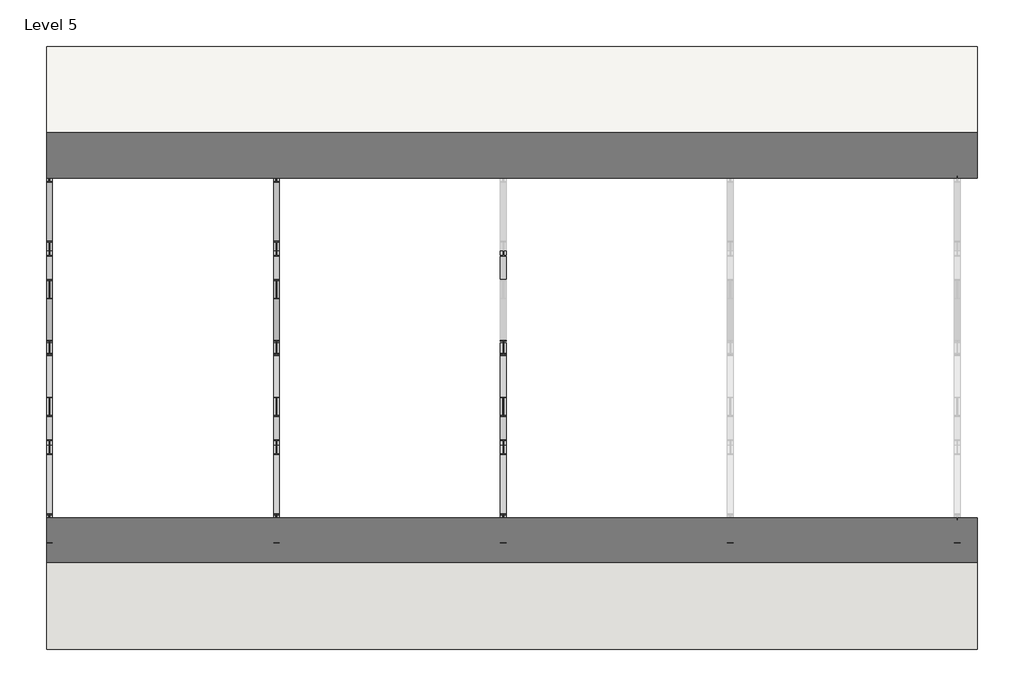
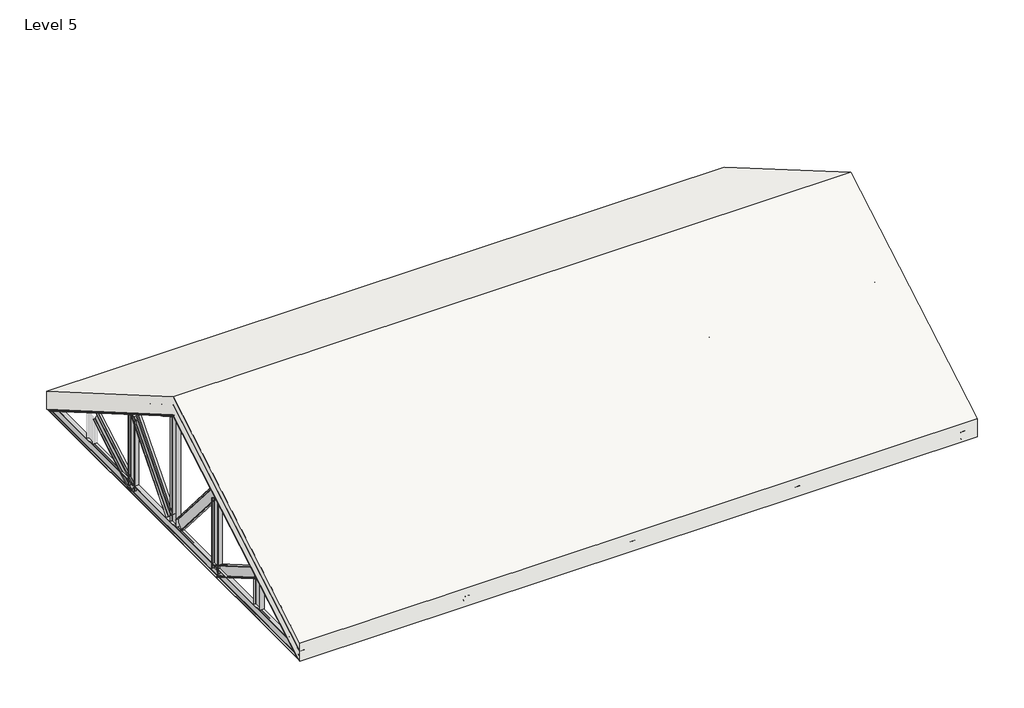
# One storey, part 1 of 2: 29 beams, 1 roof.
"""IFC4 building model written with IfcOpenShell, lengths in millimetres."""

from ifc_helpers import new_model, si_unit, frame, origin, place, context, project, spatial, polyline, circle_curve, ellipse_curve, outline, extrude, transform, mapped, element, save
from ifc_brep_helpers import plane_surface, revolved_surface, advanced_brep
from components import ub_universal_beams_ub254x102x28_e74905dc, ub_universal_beams_ub254x102x28_1dca85a9, ub_universal_beams_ub254x102x28_3582687b, ub_universal_beams_ub254x102x28_9eef3cd1, ub_universal_beams_ub254x102x28_f7ef6108, ub_universal_beams_ub254x102x28_93a23aa5, ub_universal_beams_ub254x102x28_1ec9d6d8, ub_universal_beams_ub254x102x28_a06fb1b7

model = new_model("IFC4")

# Units and contexts
model_context = context("Model", 3, world=origin())
ifc_project = project(units=[si_unit("LENGTHUNIT", "METRE", prefix="MILLI")], contexts=[model_context])

# Site, building, storey
site = spatial("IfcSite", under=ifc_project)
building = spatial("IfcBuilding", under=site)
storey = spatial("IfcBuildingStorey", under=building, Name="Level 5", Elevation=9144.0)

# Beams
placement = place(None, origin())
element("IfcBeam", 1, ObjectType="UB-Universal Beams : UB254x102x28", at=placement, inside=storey, context=model_context, shape_type="AdvancedBrep", body=[
    advanced_brep(
    [(-8879.5620752, 9795.4298445, 9040.0618528), (-8879.5620752, 9790.4089662, 9031.4136864), (-8981.7620752, 9790.4089662, 9031.4136864), (-8981.7620752, 9795.4298445, 9040.0618528), (-8941.4120752, 9795.4298445, 9040.0618528), (-8933.8120752, 9799.245712, 9046.6344592), (-8933.8120752, 9912.3158911, 9241.3911653), (-8941.4120752, 9916.1317586, 9247.9637718), (-8981.7620752, 9916.1317586, 9247.9637718), (-8981.7620752, 9921.1526369, 9256.6119381), (-8879.5620752, 9921.1526369, 9256.6119381), (-8879.5620752, 9916.1317586, 9247.9637718), (-8919.9120752, 9916.1317586, 9247.9637718), (-8927.5120752, 9912.3158911, 9241.3911653), (-8927.5120752, 9799.245712, 9046.6344592), (-8919.9120752, 9795.4298445, 9040.0618528), (-8919.9120752, 4605.8028699, 12053.0109991), (-8879.5620752, 4605.8028699, 12053.0109991), (-8927.5120752, 4605.8028699, 12061.7989892), (-8927.5120752, 4605.8028699, 12322.2010108), (-8919.9120752, 4605.8028699, 12330.9890009), (-8879.5620752, 4605.8028699, 12330.9890009), (-8879.5620752, 4605.8028699, 12342.5521457), (-8981.7620752, 4605.8028699, 12342.5521457), (-8981.7620752, 4605.8028699, 12330.9890009), (-8941.4120752, 4605.8028699, 12330.9890009), (-8933.8120752, 4605.8028699, 12322.2010108), (-8933.8120752, 4605.8028699, 12061.7989892), (-8941.4120752, 4605.8028699, 12053.0109991), (-8981.7620752, 4605.8028699, 12053.0109991), (-8981.7620752, 4605.8028699, 12041.4478543), (-8879.5620752, 4605.8028699, 12041.4478543)],
    [
        (0, 1),
        (1, 2),
        (2, 3),
        (3, 4),
        (4, 5, circle_curve(frame((-8941.4120752, 9799.245712, 9046.6344592), z_axis=(0.0, -0.8648166348106393, 0.5020878291243489), x_axis=(-1.0, 0.0, 0.0)), 7.6)),
        (5, 6),
        (6, 7, circle_curve(frame((-8941.4120752, 9912.3158911, 9241.3911653), z_axis=(0.0, -0.8648166348106393, 0.5020878291243489), x_axis=(-1.0, 0.0, 0.0)), 7.6)),
        (7, 8),
        (8, 9),
        (9, 10),
        (10, 11),
        (11, 12),
        (12, 13, circle_curve(frame((-8919.9120752, 9912.3158911, 9241.3911653), z_axis=(0.0, -0.8648166348106393, 0.5020878291243489), x_axis=(-1.0, 0.0, 0.0)), 7.6)),
        (13, 14),
        (14, 15, circle_curve(frame((-8919.9120752, 9799.245712, 9046.6344592), z_axis=(0.0, -0.8648166348106393, 0.5020878291243489), x_axis=(-1.0, 0.0, 0.0)), 7.6)),
        (15, 0),
        (16, 17),
        (17, 0),
        (15, 16),
        (18, 16, ellipse_curve(frame((-8919.9120752, 4605.8028699, 12061.7989892), z_axis=(0.0, -1.0, 0.0), x_axis=(0.0, 0.0, -1.0)), 8.7879901, 7.6)),
        (14, 18),
        (19, 18),
        (13, 19),
        (20, 19, ellipse_curve(frame((-8919.9120752, 4605.8028699, 12322.2010108), z_axis=(0.0, -1.0, 0.0), x_axis=(0.0, 0.0, -1.0)), 8.7879901, 7.6)),
        (12, 20),
        (21, 20),
        (11, 21),
        (22, 21),
        (10, 22),
        (23, 22),
        (9, 23),
        (24, 23),
        (8, 24),
        (25, 24),
        (7, 25),
        (26, 25, ellipse_curve(frame((-8941.4120752, 4605.8028699, 12322.2010108), z_axis=(0.0, -1.0, 0.0), x_axis=(0.0, 0.0, -1.0)), 8.7879901, 7.6)),
        (6, 26),
        (27, 26),
        (5, 27),
        (28, 27, ellipse_curve(frame((-8941.4120752, 4605.8028699, 12061.7989892), z_axis=(0.0, -1.0, 0.0), x_axis=(0.0, 0.0, -1.0)), 8.7879901, 7.6)),
        (4, 28),
        (29, 28),
        (3, 29),
        (30, 29),
        (2, 30),
        (31, 30),
        (1, 31),
        (17, 31),
    ],
    [
        plane_surface(frame((-8930.6620752, 9855.7808016, 9144.0128123), z_axis=(0.0, 0.8648166348106393, -0.5020878291243489), x_axis=(0.0, 0.5020878291243489, 0.8648166348106393))),
        plane_surface(frame((-8879.5620752, 4545.4739812, 12088.0362282), z_axis=(0.0, 0.5020878291243489, 0.8648166348106393), x_axis=(0.0, 0.8648166348106393, -0.5020878291243489))),
        revolved_surface(polyline([(-8927.5120752, 9799.245712003027, 9046.634459205212), (-8927.5120752, 4601.987002407376, 12064.01437289046)]), (-8919.9120752, 4549.2898487, 12094.6088347), (0.0, 0.8648166348106393, -0.5020878291243489)),
        plane_surface(frame((-8927.5120752, 4549.2898487, 12094.6088347), z_axis=(1.0, 0.0, 0.0), x_axis=(0.0, 0.8648166348106393, -0.5020878291243489))),
        revolved_surface(polyline([(-8927.5120752, 9912.315891103026, 9241.391165305211), (-8927.5120752, 4601.987002367825, 12324.416394422336)]), (-8919.9120752, 4662.3600278, 12289.3655408), (0.0, 0.8648166348106393, -0.5020878291243489)),
        plane_surface(frame((-8919.9120752, 4666.1758953, 12295.9381472), z_axis=(0.0, -0.5020878291243489, -0.8648166348106393), x_axis=(0.0, 0.8648166348106393, -0.5020878291243489))),
        plane_surface(frame((-8879.5620752, 4666.1758953, 12295.9381472), z_axis=(1.0, 0.0, 0.0), x_axis=(0.0, 0.8648166348106393, -0.5020878291243489))),
        plane_surface(frame((-8879.5620752, 4671.1967736, 12304.5863136), z_axis=(0.0, 0.5020878291243489, 0.8648166348106393), x_axis=(0.0, 0.8648166348106393, -0.5020878291243489))),
        plane_surface(frame((-8981.7620752, 4671.1967736, 12304.5863136), z_axis=(-1.0, 0.0, 0.0), x_axis=(0.0, 0.8648166348106393, -0.5020878291243489))),
        plane_surface(frame((-8981.7620752, 4666.1758953, 12295.9381472), z_axis=(0.0, -0.5020878291243489, -0.8648166348106393), x_axis=(0.0, 0.8648166348106393, -0.5020878291243489))),
        revolved_surface(polyline([(-8949.0120752, 9912.315891103026, 9241.391165305211), (-8949.0120752, 4601.987002367825, 12324.416394422336)]), (-8941.4120752, 4662.3600278, 12289.3655408), (0.0, 0.8648166348106393, -0.5020878291243489)),
        plane_surface(frame((-8933.8120752, 4662.3600278, 12289.3655408), z_axis=(-1.0, 0.0, 0.0), x_axis=(0.0, 0.8648166348106393, -0.5020878291243489))),
        revolved_surface(polyline([(-8949.0120752, 9799.245712003027, 9046.634459205212), (-8949.0120752, 4601.987002407376, 12064.01437289046)]), (-8941.4120752, 4549.2898487, 12094.6088347), (0.0, 0.8648166348106393, -0.5020878291243489)),
        plane_surface(frame((-8941.4120752, 4545.4739812, 12088.0362282), z_axis=(0.0, 0.5020878291243489, 0.8648166348106393), x_axis=(0.0, 0.8648166348106393, -0.5020878291243489))),
        plane_surface(frame((-8981.7620752, 4545.4739812, 12088.0362282), z_axis=(-1.0, 0.0, 0.0), x_axis=(0.0, 0.8648166348106393, -0.5020878291243489))),
        plane_surface(frame((-8981.7620752, 4540.4531029, 12079.3880619), z_axis=(0.0, -0.5020878291243489, -0.8648166348106393), x_axis=(0.0, 0.8648166348106393, -0.5020878291243489))),
        plane_surface(frame((-8879.5620752, 4540.4531029, 12079.3880619), z_axis=(1.0, 0.0, 0.0), x_axis=(0.0, 0.8648166348106393, -0.5020878291243489))),
        plane_surface(frame((-8930.6620752, 4605.8028699, 12342.5521457), z_axis=(0.0, -1.0, 0.0), x_axis=(0.0, 0.0, 1.0))),
    ],
    [
        (0, [[1, 2, 3, 4, 5, 6, 7, 8, 9, 10, 11, 12, 13, 14, 15, 16]]),
        (1, [[17, 18, -16, 19]]),
        (2, [[20, -19, -15, 21]]),
        (3, [[22, -21, -14, 23]]),
        (4, [[24, -23, -13, 25]]),
        (5, [[26, -25, -12, 27]]),
        (6, [[28, -27, -11, 29]]),
        (7, [[30, -29, -10, 31]]),
        (8, [[32, -31, -9, 33]]),
        (9, [[34, -33, -8, 35]]),
        (10, [[36, -35, -7, 37]]),
        (11, [[38, -37, -6, 39]]),
        (12, [[40, -39, -5, 41]]),
        (13, [[42, -41, -4, 43]]),
        (14, [[44, -43, -3, 45]]),
        (15, [[46, -45, -2, 47]]),
        (16, [[48, -47, -1, -18]]),
        (17, [[-17, -20, -22, -24, -26, -28, -30, -32, -34, -36, -38, -40, -42, -44, -46, -48]]),
    ],
),
])
element("IfcBeam", 2, ObjectType="UB-Universal Beams : UB254x102x28", at=placement, inside=storey, context=model_context, shape_type="AdvancedBrep", body=[
    advanced_brep(
    [(-8879.5620752, -583.8241047, 9040.0618528), (-8919.9120752, -583.8241047, 9040.0618528), (-8927.5120752, -587.6399722, 9046.6344592), (-8927.5120752, -700.7101513, 9241.3911653), (-8919.9120752, -704.5260188, 9247.9637718), (-8879.5620752, -704.5260188, 9247.9637718), (-8879.5620752, -709.5468971, 9256.6119381), (-8981.7620752, -709.5468971, 9256.6119381), (-8981.7620752, -704.5260188, 9247.9637718), (-8941.4120752, -704.5260188, 9247.9637718), (-8933.8120752, -700.7101513, 9241.3911653), (-8933.8120752, -587.6399722, 9046.6344592), (-8941.4120752, -583.8241047, 9040.0618528), (-8981.7620752, -583.8241047, 9040.0618528), (-8981.7620752, -578.8032264, 9031.4136864), (-8879.5620752, -578.8032264, 9031.4136864), (-8879.5620752, 4605.8028699, 12053.0109991), (-8919.9120752, 4605.8028699, 12053.0109991), (-8927.5120752, 4605.8028699, 12061.7989892), (-8927.5120752, 4605.8028699, 12322.2010108), (-8919.9120752, 4605.8028699, 12330.9890009), (-8879.5620752, 4605.8028699, 12330.9890009), (-8879.5620752, 4605.8028699, 12342.5521457), (-8981.7620752, 4605.8028699, 12342.5521457), (-8981.7620752, 4605.8028699, 12330.9890009), (-8941.4120752, 4605.8028699, 12330.9890009), (-8933.8120752, 4605.8028699, 12322.2010108), (-8933.8120752, 4605.8028699, 12061.7989892), (-8941.4120752, 4605.8028699, 12053.0109991), (-8981.7620752, 4605.8028699, 12053.0109991), (-8981.7620752, 4605.8028699, 12041.4478543), (-8879.5620752, 4605.8028699, 12041.4478543)],
    [
        (0, 1),
        (1, 2, circle_curve(frame((-8919.9120752, -587.6399722, 9046.6344592), z_axis=(0.0, 0.8648166348106395, 0.5020878291243485), x_axis=(-1.0, 0.0, 0.0)), 7.6)),
        (2, 3),
        (3, 4, circle_curve(frame((-8919.9120752, -700.7101513, 9241.3911653), z_axis=(0.0, 0.8648166348106395, 0.5020878291243485), x_axis=(-1.0, 0.0, 0.0)), 7.6)),
        (4, 5),
        (5, 6),
        (6, 7),
        (7, 8),
        (8, 9),
        (9, 10, circle_curve(frame((-8941.4120752, -700.7101513, 9241.3911653), z_axis=(0.0, 0.8648166348106395, 0.5020878291243485), x_axis=(-1.0, 0.0, 0.0)), 7.6)),
        (10, 11),
        (11, 12, circle_curve(frame((-8941.4120752, -587.6399722, 9046.6344592), z_axis=(0.0, 0.8648166348106395, 0.5020878291243485), x_axis=(-1.0, 0.0, 0.0)), 7.6)),
        (12, 13),
        (13, 14),
        (14, 15),
        (15, 0),
        (0, 16),
        (16, 17),
        (17, 1),
        (17, 18, ellipse_curve(frame((-8919.9120752, 4605.8028699, 12061.7989892), z_axis=(0.0, 1.0, 0.0), x_axis=(0.0, 0.0, 1.0)), 8.7879901, 7.6)),
        (18, 2),
        (18, 19),
        (19, 3),
        (19, 20, ellipse_curve(frame((-8919.9120752, 4605.8028699, 12322.2010108), z_axis=(0.0, 1.0, 0.0), x_axis=(0.0, 0.0, 1.0)), 8.7879901, 7.6)),
        (20, 4),
        (20, 21),
        (21, 5),
        (21, 22),
        (22, 6),
        (22, 23),
        (23, 7),
        (23, 24),
        (24, 8),
        (24, 25),
        (25, 9),
        (25, 26, ellipse_curve(frame((-8941.4120752, 4605.8028699, 12322.2010108), z_axis=(0.0, 1.0, 0.0), x_axis=(0.0, 0.0, 1.0)), 8.7879901, 7.6)),
        (26, 10),
        (26, 27),
        (27, 11),
        (27, 28, ellipse_curve(frame((-8941.4120752, 4605.8028699, 12061.7989892), z_axis=(0.0, 1.0, 0.0), x_axis=(0.0, 0.0, 1.0)), 8.7879901, 7.6)),
        (28, 12),
        (28, 29),
        (29, 13),
        (29, 30),
        (30, 14),
        (30, 31),
        (31, 15),
        (31, 16),
    ],
    [
        plane_surface(frame((-8930.6620752, -644.1750617, 9144.0128123), z_axis=(0.0, -0.8648166348106395, -0.5020878291243485), x_axis=(0.0, -0.5020878291243485, 0.8648166348106395))),
        plane_surface(frame((-8879.5620752, -583.8241047, 9040.0618528), z_axis=(0.0, -0.5020878291243485, 0.8648166348106395), x_axis=(0.0, 0.8648166348106395, 0.5020878291243485))),
        revolved_surface(polyline([(-8927.5120752, 4609.618737395652, 12064.014372885247), (-8927.5120752, -587.6399722, 9046.6344592)]), (-8919.9120752, -587.6399722, 9046.6344592), (0.0, 0.8648166348106395, 0.5020878291243485)),
        plane_surface(frame((-8927.5120752, -587.6399722, 9046.6344592), z_axis=(1.0, 0.0, 0.0), x_axis=(0.0, 0.8648166348106395, 0.5020878291243485))),
        revolved_surface(polyline([(-8927.5120752, 4609.618737435201, 12324.416394417123), (-8927.5120752, -700.7101513, 9241.3911653)]), (-8919.9120752, -700.7101513, 9241.3911653), (0.0, 0.8648166348106395, 0.5020878291243485)),
        plane_surface(frame((-8919.9120752, -704.5260188, 9247.9637718), z_axis=(0.0, 0.5020878291243485, -0.8648166348106395), x_axis=(0.0, 0.8648166348106395, 0.5020878291243485))),
        plane_surface(frame((-8879.5620752, -704.5260188, 9247.9637718), z_axis=(1.0, 0.0, 0.0), x_axis=(0.0, 0.8648166348106395, 0.5020878291243485))),
        plane_surface(frame((-8879.5620752, -709.5468971, 9256.6119381), z_axis=(0.0, -0.5020878291243485, 0.8648166348106395), x_axis=(0.0, 0.8648166348106395, 0.5020878291243485))),
        plane_surface(frame((-8981.7620752, -709.5468971, 9256.6119381), z_axis=(-1.0, 0.0, 0.0), x_axis=(0.0, 0.8648166348106395, 0.5020878291243485))),
        plane_surface(frame((-8981.7620752, -704.5260188, 9247.9637718), z_axis=(0.0, 0.5020878291243485, -0.8648166348106395), x_axis=(0.0, 0.8648166348106395, 0.5020878291243485))),
        revolved_surface(polyline([(-8949.0120752, 4609.618737435201, 12324.416394417123), (-8949.0120752, -700.7101513, 9241.3911653)]), (-8941.4120752, -700.7101513, 9241.3911653), (0.0, 0.8648166348106395, 0.5020878291243485)),
        plane_surface(frame((-8933.8120752, -700.7101513, 9241.3911653), z_axis=(-1.0, 0.0, 0.0), x_axis=(0.0, 0.8648166348106395, 0.5020878291243485))),
        revolved_surface(polyline([(-8949.0120752, 4609.618737395652, 12064.014372885247), (-8949.0120752, -587.6399722, 9046.6344592)]), (-8941.4120752, -587.6399722, 9046.6344592), (0.0, 0.8648166348106395, 0.5020878291243485)),
        plane_surface(frame((-8941.4120752, -583.8241047, 9040.0618528), z_axis=(0.0, -0.5020878291243485, 0.8648166348106395), x_axis=(0.0, 0.8648166348106395, 0.5020878291243485))),
        plane_surface(frame((-8981.7620752, -583.8241047, 9040.0618528), z_axis=(-1.0, 0.0, 0.0), x_axis=(0.0, 0.8648166348106395, 0.5020878291243485))),
        plane_surface(frame((-8981.7620752, -578.8032264, 9031.4136864), z_axis=(0.0, 0.5020878291243485, -0.8648166348106395), x_axis=(0.0, 0.8648166348106395, 0.5020878291243485))),
        plane_surface(frame((-8879.5620752, -578.8032264, 9031.4136864), z_axis=(1.0, 0.0, 0.0), x_axis=(0.0, 0.8648166348106395, 0.5020878291243485))),
        plane_surface(frame((-8930.6620752, 4605.8028699, 12342.5521457), z_axis=(0.0, 1.0, 0.0), x_axis=(0.0, 0.0, -1.0))),
    ],
    [
        (0, [[1, 2, 3, 4, 5, 6, 7, 8, 9, 10, 11, 12, 13, 14, 15, 16]]),
        (1, [[-1, 17, 18, 19]]),
        (2, [[-2, -19, 20, 21]]),
        (3, [[-3, -21, 22, 23]]),
        (4, [[-4, -23, 24, 25]]),
        (5, [[-5, -25, 26, 27]]),
        (6, [[-6, -27, 28, 29]]),
        (7, [[-7, -29, 30, 31]]),
        (8, [[-8, -31, 32, 33]]),
        (9, [[-9, -33, 34, 35]]),
        (10, [[-10, -35, 36, 37]]),
        (11, [[-11, -37, 38, 39]]),
        (12, [[-12, -39, 40, 41]]),
        (13, [[-13, -41, 42, 43]]),
        (14, [[-14, -43, 44, 45]]),
        (15, [[-15, -45, 46, 47]]),
        (16, [[-16, -47, 48, -17]]),
        (17, [[-48, -46, -44, -42, -40, -38, -36, -34, -32, -30, -28, -26, -24, -22, -20, -18]]),
    ],
),
])
element("IfcBeam", 3, ObjectType="UB-Universal Beams : UB254x102x28", at=placement, inside=storey, context=model_context, shape_type="AdvancedBrep", body=[
    advanced_brep(
    [(-4879.5620752, 9795.4298445, 9040.0618528), (-4879.5620752, 9790.4089662, 9031.4136864), (-4981.7620752, 9790.4089662, 9031.4136864), (-4981.7620752, 9795.4298445, 9040.0618528), (-4941.4120752, 9795.4298445, 9040.0618528), (-4933.8120752, 9799.245712, 9046.6344592), (-4933.8120752, 9912.3158911, 9241.3911653), (-4941.4120752, 9916.1317586, 9247.9637718), (-4981.7620752, 9916.1317586, 9247.9637718), (-4981.7620752, 9921.1526369, 9256.6119381), (-4879.5620752, 9921.1526369, 9256.6119381), (-4879.5620752, 9916.1317586, 9247.9637718), (-4919.9120752, 9916.1317586, 9247.9637718), (-4927.5120752, 9912.3158911, 9241.3911653), (-4927.5120752, 9799.245712, 9046.6344592), (-4919.9120752, 9795.4298445, 9040.0618528), (-4919.9120752, 4605.8028699, 12053.0109991), (-4879.5620752, 4605.8028699, 12053.0109991), (-4927.5120752, 4605.8028699, 12061.7989892), (-4927.5120752, 4605.8028699, 12322.2010108), (-4919.9120752, 4605.8028699, 12330.9890009), (-4879.5620752, 4605.8028699, 12330.9890009), (-4879.5620752, 4605.8028699, 12342.5521457), (-4981.7620752, 4605.8028699, 12342.5521457), (-4981.7620752, 4605.8028699, 12330.9890009), (-4941.4120752, 4605.8028699, 12330.9890009), (-4933.8120752, 4605.8028699, 12322.2010108), (-4933.8120752, 4605.8028699, 12061.7989892), (-4941.4120752, 4605.8028699, 12053.0109991), (-4981.7620752, 4605.8028699, 12053.0109991), (-4981.7620752, 4605.8028699, 12041.4478543), (-4879.5620752, 4605.8028699, 12041.4478543)],
    [
        (0, 1),
        (1, 2),
        (2, 3),
        (3, 4),
        (4, 5, circle_curve(frame((-4941.4120752, 9799.245712, 9046.6344592), z_axis=(0.0, -0.8648166348106393, 0.5020878291243489), x_axis=(-1.0, 0.0, 0.0)), 7.6)),
        (5, 6),
        (6, 7, circle_curve(frame((-4941.4120752, 9912.3158911, 9241.3911653), z_axis=(0.0, -0.8648166348106393, 0.5020878291243489), x_axis=(-1.0, 0.0, 0.0)), 7.6)),
        (7, 8),
        (8, 9),
        (9, 10),
        (10, 11),
        (11, 12),
        (12, 13, circle_curve(frame((-4919.9120752, 9912.3158911, 9241.3911653), z_axis=(0.0, -0.8648166348106393, 0.5020878291243489), x_axis=(-1.0, 0.0, 0.0)), 7.6)),
        (13, 14),
        (14, 15, circle_curve(frame((-4919.9120752, 9799.245712, 9046.6344592), z_axis=(0.0, -0.8648166348106393, 0.5020878291243489), x_axis=(-1.0, 0.0, 0.0)), 7.6)),
        (15, 0),
        (16, 17),
        (17, 0),
        (15, 16),
        (18, 16, ellipse_curve(frame((-4919.9120752, 4605.8028699, 12061.7989892), z_axis=(0.0, -1.0, 0.0), x_axis=(0.0, 0.0, -1.0)), 8.7879901, 7.6)),
        (14, 18),
        (19, 18),
        (13, 19),
        (20, 19, ellipse_curve(frame((-4919.9120752, 4605.8028699, 12322.2010108), z_axis=(0.0, -1.0, 0.0), x_axis=(0.0, 0.0, -1.0)), 8.7879901, 7.6)),
        (12, 20),
        (21, 20),
        (11, 21),
        (22, 21),
        (10, 22),
        (23, 22),
        (9, 23),
        (24, 23),
        (8, 24),
        (25, 24),
        (7, 25),
        (26, 25, ellipse_curve(frame((-4941.4120752, 4605.8028699, 12322.2010108), z_axis=(0.0, -1.0, 0.0), x_axis=(0.0, 0.0, -1.0)), 8.7879901, 7.6)),
        (6, 26),
        (27, 26),
        (5, 27),
        (28, 27, ellipse_curve(frame((-4941.4120752, 4605.8028699, 12061.7989892), z_axis=(0.0, -1.0, 0.0), x_axis=(0.0, 0.0, -1.0)), 8.7879901, 7.6)),
        (4, 28),
        (29, 28),
        (3, 29),
        (30, 29),
        (2, 30),
        (31, 30),
        (1, 31),
        (17, 31),
    ],
    [
        plane_surface(frame((-4930.6620752, 9855.7808016, 9144.0128123), z_axis=(0.0, 0.8648166348106393, -0.5020878291243489), x_axis=(0.0, 0.5020878291243489, 0.8648166348106393))),
        plane_surface(frame((-4879.5620752, 4545.4739812, 12088.0362282), z_axis=(0.0, 0.5020878291243489, 0.8648166348106393), x_axis=(0.0, 0.8648166348106393, -0.5020878291243489))),
        revolved_surface(polyline([(-4927.5120752, 9799.245712003027, 9046.634459205212), (-4927.5120752, 4601.987002407376, 12064.01437289046)]), (-4919.9120752, 4549.2898487, 12094.6088347), (0.0, 0.8648166348106393, -0.5020878291243489)),
        plane_surface(frame((-4927.5120752, 4549.2898487, 12094.6088347), z_axis=(1.0, 0.0, 0.0), x_axis=(0.0, 0.8648166348106393, -0.5020878291243489))),
        revolved_surface(polyline([(-4927.5120752, 9912.315891103026, 9241.391165305211), (-4927.5120752, 4601.987002367825, 12324.416394422336)]), (-4919.9120752, 4662.3600278, 12289.3655408), (0.0, 0.8648166348106393, -0.5020878291243489)),
        plane_surface(frame((-4919.9120752, 4666.1758953, 12295.9381472), z_axis=(0.0, -0.5020878291243489, -0.8648166348106393), x_axis=(0.0, 0.8648166348106393, -0.5020878291243489))),
        plane_surface(frame((-4879.5620752, 4666.1758953, 12295.9381472), z_axis=(1.0, 0.0, 0.0), x_axis=(0.0, 0.8648166348106393, -0.5020878291243489))),
        plane_surface(frame((-4879.5620752, 4671.1967736, 12304.5863136), z_axis=(0.0, 0.5020878291243489, 0.8648166348106393), x_axis=(0.0, 0.8648166348106393, -0.5020878291243489))),
        plane_surface(frame((-4981.7620752, 4671.1967736, 12304.5863136), z_axis=(-1.0, 0.0, 0.0), x_axis=(0.0, 0.8648166348106393, -0.5020878291243489))),
        plane_surface(frame((-4981.7620752, 4666.1758953, 12295.9381472), z_axis=(0.0, -0.5020878291243489, -0.8648166348106393), x_axis=(0.0, 0.8648166348106393, -0.5020878291243489))),
        revolved_surface(polyline([(-4949.0120752, 9912.315891103026, 9241.391165305211), (-4949.0120752, 4601.987002367825, 12324.416394422336)]), (-4941.4120752, 4662.3600278, 12289.3655408), (0.0, 0.8648166348106393, -0.5020878291243489)),
        plane_surface(frame((-4933.8120752, 4662.3600278, 12289.3655408), z_axis=(-1.0, 0.0, 0.0), x_axis=(0.0, 0.8648166348106393, -0.5020878291243489))),
        revolved_surface(polyline([(-4949.0120752, 9799.245712003027, 9046.634459205212), (-4949.0120752, 4601.987002407376, 12064.01437289046)]), (-4941.4120752, 4549.2898487, 12094.6088347), (0.0, 0.8648166348106393, -0.5020878291243489)),
        plane_surface(frame((-4941.4120752, 4545.4739812, 12088.0362282), z_axis=(0.0, 0.5020878291243489, 0.8648166348106393), x_axis=(0.0, 0.8648166348106393, -0.5020878291243489))),
        plane_surface(frame((-4981.7620752, 4545.4739812, 12088.0362282), z_axis=(-1.0, 0.0, 0.0), x_axis=(0.0, 0.8648166348106393, -0.5020878291243489))),
        plane_surface(frame((-4981.7620752, 4540.4531029, 12079.3880619), z_axis=(0.0, -0.5020878291243489, -0.8648166348106393), x_axis=(0.0, 0.8648166348106393, -0.5020878291243489))),
        plane_surface(frame((-4879.5620752, 4540.4531029, 12079.3880619), z_axis=(1.0, 0.0, 0.0), x_axis=(0.0, 0.8648166348106393, -0.5020878291243489))),
        plane_surface(frame((-4930.6620752, 4605.8028699, 12342.5521457), z_axis=(0.0, -1.0, 0.0), x_axis=(0.0, 0.0, 1.0))),
    ],
    [
        (0, [[1, 2, 3, 4, 5, 6, 7, 8, 9, 10, 11, 12, 13, 14, 15, 16]]),
        (1, [[17, 18, -16, 19]]),
        (2, [[20, -19, -15, 21]]),
        (3, [[22, -21, -14, 23]]),
        (4, [[24, -23, -13, 25]]),
        (5, [[26, -25, -12, 27]]),
        (6, [[28, -27, -11, 29]]),
        (7, [[30, -29, -10, 31]]),
        (8, [[32, -31, -9, 33]]),
        (9, [[34, -33, -8, 35]]),
        (10, [[36, -35, -7, 37]]),
        (11, [[38, -37, -6, 39]]),
        (12, [[40, -39, -5, 41]]),
        (13, [[42, -41, -4, 43]]),
        (14, [[44, -43, -3, 45]]),
        (15, [[46, -45, -2, 47]]),
        (16, [[48, -47, -1, -18]]),
        (17, [[-17, -20, -22, -24, -26, -28, -30, -32, -34, -36, -38, -40, -42, -44, -46, -48]]),
    ],
),
])
element("IfcBeam", 4, ObjectType="UB-Universal Beams : UB254x102x28", at=placement, inside=storey, context=model_context, shape_type="AdvancedBrep", body=[
    advanced_brep(
    [(-4879.5620752, -583.8241047, 9040.0618528), (-4919.9120752, -583.8241047, 9040.0618528), (-4927.5120752, -587.6399722, 9046.6344592), (-4927.5120752, -700.7101513, 9241.3911653), (-4919.9120752, -704.5260188, 9247.9637718), (-4879.5620752, -704.5260188, 9247.9637718), (-4879.5620752, -709.5468971, 9256.6119381), (-4981.7620752, -709.5468971, 9256.6119381), (-4981.7620752, -704.5260188, 9247.9637718), (-4941.4120752, -704.5260188, 9247.9637718), (-4933.8120752, -700.7101513, 9241.3911653), (-4933.8120752, -587.6399722, 9046.6344592), (-4941.4120752, -583.8241047, 9040.0618528), (-4981.7620752, -583.8241047, 9040.0618528), (-4981.7620752, -578.8032264, 9031.4136864), (-4879.5620752, -578.8032264, 9031.4136864), (-4879.5620752, 4605.8028699, 12053.0109991), (-4919.9120752, 4605.8028699, 12053.0109991), (-4927.5120752, 4605.8028699, 12061.7989892), (-4927.5120752, 4605.8028699, 12322.2010108), (-4919.9120752, 4605.8028699, 12330.9890009), (-4879.5620752, 4605.8028699, 12330.9890009), (-4879.5620752, 4605.8028699, 12342.5521457), (-4981.7620752, 4605.8028699, 12342.5521457), (-4981.7620752, 4605.8028699, 12330.9890009), (-4941.4120752, 4605.8028699, 12330.9890009), (-4933.8120752, 4605.8028699, 12322.2010108), (-4933.8120752, 4605.8028699, 12061.7989892), (-4941.4120752, 4605.8028699, 12053.0109991), (-4981.7620752, 4605.8028699, 12053.0109991), (-4981.7620752, 4605.8028699, 12041.4478543), (-4879.5620752, 4605.8028699, 12041.4478543)],
    [
        (0, 1),
        (1, 2, circle_curve(frame((-4919.9120752, -587.6399722, 9046.6344592), z_axis=(0.0, 0.8648166348106395, 0.5020878291243485), x_axis=(-1.0, 0.0, 0.0)), 7.6)),
        (2, 3),
        (3, 4, circle_curve(frame((-4919.9120752, -700.7101513, 9241.3911653), z_axis=(0.0, 0.8648166348106395, 0.5020878291243485), x_axis=(-1.0, 0.0, 0.0)), 7.6)),
        (4, 5),
        (5, 6),
        (6, 7),
        (7, 8),
        (8, 9),
        (9, 10, circle_curve(frame((-4941.4120752, -700.7101513, 9241.3911653), z_axis=(0.0, 0.8648166348106395, 0.5020878291243485), x_axis=(-1.0, 0.0, 0.0)), 7.6)),
        (10, 11),
        (11, 12, circle_curve(frame((-4941.4120752, -587.6399722, 9046.6344592), z_axis=(0.0, 0.8648166348106395, 0.5020878291243485), x_axis=(-1.0, 0.0, 0.0)), 7.6)),
        (12, 13),
        (13, 14),
        (14, 15),
        (15, 0),
        (0, 16),
        (16, 17),
        (17, 1),
        (17, 18, ellipse_curve(frame((-4919.9120752, 4605.8028699, 12061.7989892), z_axis=(0.0, 1.0, 0.0), x_axis=(0.0, 0.0, 1.0)), 8.7879901, 7.6)),
        (18, 2),
        (18, 19),
        (19, 3),
        (19, 20, ellipse_curve(frame((-4919.9120752, 4605.8028699, 12322.2010108), z_axis=(0.0, 1.0, 0.0), x_axis=(0.0, 0.0, 1.0)), 8.7879901, 7.6)),
        (20, 4),
        (20, 21),
        (21, 5),
        (21, 22),
        (22, 6),
        (22, 23),
        (23, 7),
        (23, 24),
        (24, 8),
        (24, 25),
        (25, 9),
        (25, 26, ellipse_curve(frame((-4941.4120752, 4605.8028699, 12322.2010108), z_axis=(0.0, 1.0, 0.0), x_axis=(0.0, 0.0, 1.0)), 8.7879901, 7.6)),
        (26, 10),
        (26, 27),
        (27, 11),
        (27, 28, ellipse_curve(frame((-4941.4120752, 4605.8028699, 12061.7989892), z_axis=(0.0, 1.0, 0.0), x_axis=(0.0, 0.0, 1.0)), 8.7879901, 7.6)),
        (28, 12),
        (28, 29),
        (29, 13),
        (29, 30),
        (30, 14),
        (30, 31),
        (31, 15),
        (31, 16),
    ],
    [
        plane_surface(frame((-4930.6620752, -644.1750617, 9144.0128123), z_axis=(0.0, -0.8648166348106395, -0.5020878291243485), x_axis=(0.0, -0.5020878291243485, 0.8648166348106395))),
        plane_surface(frame((-4879.5620752, -583.8241047, 9040.0618528), z_axis=(0.0, -0.5020878291243485, 0.8648166348106395), x_axis=(0.0, 0.8648166348106395, 0.5020878291243485))),
        revolved_surface(polyline([(-4927.5120752, 4609.618737395652, 12064.014372885247), (-4927.5120752, -587.6399722, 9046.6344592)]), (-4919.9120752, -587.6399722, 9046.6344592), (0.0, 0.8648166348106395, 0.5020878291243485)),
        plane_surface(frame((-4927.5120752, -587.6399722, 9046.6344592), z_axis=(1.0, 0.0, 0.0), x_axis=(0.0, 0.8648166348106395, 0.5020878291243485))),
        revolved_surface(polyline([(-4927.5120752, 4609.618737435201, 12324.416394417123), (-4927.5120752, -700.7101513, 9241.3911653)]), (-4919.9120752, -700.7101513, 9241.3911653), (0.0, 0.8648166348106395, 0.5020878291243485)),
        plane_surface(frame((-4919.9120752, -704.5260188, 9247.9637718), z_axis=(0.0, 0.5020878291243485, -0.8648166348106395), x_axis=(0.0, 0.8648166348106395, 0.5020878291243485))),
        plane_surface(frame((-4879.5620752, -704.5260188, 9247.9637718), z_axis=(1.0, 0.0, 0.0), x_axis=(0.0, 0.8648166348106395, 0.5020878291243485))),
        plane_surface(frame((-4879.5620752, -709.5468971, 9256.6119381), z_axis=(0.0, -0.5020878291243485, 0.8648166348106395), x_axis=(0.0, 0.8648166348106395, 0.5020878291243485))),
        plane_surface(frame((-4981.7620752, -709.5468971, 9256.6119381), z_axis=(-1.0, 0.0, 0.0), x_axis=(0.0, 0.8648166348106395, 0.5020878291243485))),
        plane_surface(frame((-4981.7620752, -704.5260188, 9247.9637718), z_axis=(0.0, 0.5020878291243485, -0.8648166348106395), x_axis=(0.0, 0.8648166348106395, 0.5020878291243485))),
        revolved_surface(polyline([(-4949.0120752, 4609.618737435201, 12324.416394417123), (-4949.0120752, -700.7101513, 9241.3911653)]), (-4941.4120752, -700.7101513, 9241.3911653), (0.0, 0.8648166348106395, 0.5020878291243485)),
        plane_surface(frame((-4933.8120752, -700.7101513, 9241.3911653), z_axis=(-1.0, 0.0, 0.0), x_axis=(0.0, 0.8648166348106395, 0.5020878291243485))),
        revolved_surface(polyline([(-4949.0120752, 4609.618737395652, 12064.014372885247), (-4949.0120752, -587.6399722, 9046.6344592)]), (-4941.4120752, -587.6399722, 9046.6344592), (0.0, 0.8648166348106395, 0.5020878291243485)),
        plane_surface(frame((-4941.4120752, -583.8241047, 9040.0618528), z_axis=(0.0, -0.5020878291243485, 0.8648166348106395), x_axis=(0.0, 0.8648166348106395, 0.5020878291243485))),
        plane_surface(frame((-4981.7620752, -583.8241047, 9040.0618528), z_axis=(-1.0, 0.0, 0.0), x_axis=(0.0, 0.8648166348106395, 0.5020878291243485))),
        plane_surface(frame((-4981.7620752, -578.8032264, 9031.4136864), z_axis=(0.0, 0.5020878291243485, -0.8648166348106395), x_axis=(0.0, 0.8648166348106395, 0.5020878291243485))),
        plane_surface(frame((-4879.5620752, -578.8032264, 9031.4136864), z_axis=(1.0, 0.0, 0.0), x_axis=(0.0, 0.8648166348106395, 0.5020878291243485))),
        plane_surface(frame((-4930.6620752, 4605.8028699, 12342.5521457), z_axis=(0.0, 1.0, 0.0), x_axis=(0.0, 0.0, -1.0))),
    ],
    [
        (0, [[1, 2, 3, 4, 5, 6, 7, 8, 9, 10, 11, 12, 13, 14, 15, 16]]),
        (1, [[-1, 17, 18, 19]]),
        (2, [[-2, -19, 20, 21]]),
        (3, [[-3, -21, 22, 23]]),
        (4, [[-4, -23, 24, 25]]),
        (5, [[-5, -25, 26, 27]]),
        (6, [[-6, -27, 28, 29]]),
        (7, [[-7, -29, 30, 31]]),
        (8, [[-8, -31, 32, 33]]),
        (9, [[-9, -33, 34, 35]]),
        (10, [[-10, -35, 36, 37]]),
        (11, [[-11, -37, 38, 39]]),
        (12, [[-12, -39, 40, 41]]),
        (13, [[-13, -41, 42, 43]]),
        (14, [[-14, -43, 44, 45]]),
        (15, [[-15, -45, 46, 47]]),
        (16, [[-16, -47, 48, -17]]),
        (17, [[-48, -46, -44, -42, -40, -38, -36, -34, -32, -30, -28, -26, -24, -22, -20, -18]]),
    ],
),
])
element("IfcBeam", 5, ObjectType="UB-Universal Beams : UB254x102x28", at=placement, inside=storey, context=model_context, shape_type="AdvancedBrep", body=[
    advanced_brep(
    [(-879.5620752, -583.8241047, 9040.0618528), (-919.9120752, -583.8241047, 9040.0618528), (-927.5120752, -587.6399722, 9046.6344592), (-927.5120752, -700.7101513, 9241.3911653), (-919.9120752, -704.5260188, 9247.9637718), (-879.5620752, -704.5260188, 9247.9637718), (-879.5620752, -709.5468971, 9256.6119381), (-981.7620752, -709.5468971, 9256.6119381), (-981.7620752, -704.5260188, 9247.9637718), (-941.4120752, -704.5260188, 9247.9637718), (-933.8120752, -700.7101513, 9241.3911653), (-933.8120752, -587.6399722, 9046.6344592), (-941.4120752, -583.8241047, 9040.0618528), (-981.7620752, -583.8241047, 9040.0618528), (-981.7620752, -578.8032264, 9031.4136864), (-879.5620752, -578.8032264, 9031.4136864), (-879.5620752, 4605.8028699, 12053.0109991), (-919.9120752, 4605.8028699, 12053.0109991), (-927.5120752, 4605.8028699, 12061.7989892), (-927.5120752, 4605.8028699, 12322.2010108), (-919.9120752, 4605.8028699, 12330.9890009), (-879.5620752, 4605.8028699, 12330.9890009), (-879.5620752, 4605.8028699, 12342.5521457), (-981.7620752, 4605.8028699, 12342.5521457), (-981.7620752, 4605.8028699, 12330.9890009), (-941.4120752, 4605.8028699, 12330.9890009), (-933.8120752, 4605.8028699, 12322.2010108), (-933.8120752, 4605.8028699, 12061.7989892), (-941.4120752, 4605.8028699, 12053.0109991), (-981.7620752, 4605.8028699, 12053.0109991), (-981.7620752, 4605.8028699, 12041.4478543), (-879.5620752, 4605.8028699, 12041.4478543)],
    [
        (0, 1),
        (1, 2, circle_curve(frame((-919.9120752, -587.6399722, 9046.6344592), z_axis=(0.0, 0.8648166348106395, 0.5020878291243485), x_axis=(-1.0, 0.0, 0.0)), 7.6)),
        (2, 3),
        (3, 4, circle_curve(frame((-919.9120752, -700.7101513, 9241.3911653), z_axis=(0.0, 0.8648166348106395, 0.5020878291243485), x_axis=(-1.0, 0.0, 0.0)), 7.6)),
        (4, 5),
        (5, 6),
        (6, 7),
        (7, 8),
        (8, 9),
        (9, 10, circle_curve(frame((-941.4120752, -700.7101513, 9241.3911653), z_axis=(0.0, 0.8648166348106395, 0.5020878291243485), x_axis=(-1.0, 0.0, 0.0)), 7.6)),
        (10, 11),
        (11, 12, circle_curve(frame((-941.4120752, -587.6399722, 9046.6344592), z_axis=(0.0, 0.8648166348106395, 0.5020878291243485), x_axis=(-1.0, 0.0, 0.0)), 7.6)),
        (12, 13),
        (13, 14),
        (14, 15),
        (15, 0),
        (0, 16),
        (16, 17),
        (17, 1),
        (17, 18, ellipse_curve(frame((-919.9120752, 4605.8028699, 12061.7989892), z_axis=(0.0, 1.0, 0.0), x_axis=(0.0, 0.0, 1.0)), 8.7879901, 7.6)),
        (18, 2),
        (18, 19),
        (19, 3),
        (19, 20, ellipse_curve(frame((-919.9120752, 4605.8028699, 12322.2010108), z_axis=(0.0, 1.0, 0.0), x_axis=(0.0, 0.0, 1.0)), 8.7879901, 7.6)),
        (20, 4),
        (20, 21),
        (21, 5),
        (21, 22),
        (22, 6),
        (22, 23),
        (23, 7),
        (23, 24),
        (24, 8),
        (24, 25),
        (25, 9),
        (25, 26, ellipse_curve(frame((-941.4120752, 4605.8028699, 12322.2010108), z_axis=(0.0, 1.0, 0.0), x_axis=(0.0, 0.0, 1.0)), 8.7879901, 7.6)),
        (26, 10),
        (26, 27),
        (27, 11),
        (27, 28, ellipse_curve(frame((-941.4120752, 4605.8028699, 12061.7989892), z_axis=(0.0, 1.0, 0.0), x_axis=(0.0, 0.0, 1.0)), 8.7879901, 7.6)),
        (28, 12),
        (28, 29),
        (29, 13),
        (29, 30),
        (30, 14),
        (30, 31),
        (31, 15),
        (31, 16),
    ],
    [
        plane_surface(frame((-930.6620752, -644.1750617, 9144.0128123), z_axis=(0.0, -0.8648166348106395, -0.5020878291243485), x_axis=(0.0, -0.5020878291243485, 0.8648166348106395))),
        plane_surface(frame((-879.5620752, -583.8241047, 9040.0618528), z_axis=(0.0, -0.5020878291243485, 0.8648166348106395), x_axis=(0.0, 0.8648166348106395, 0.5020878291243485))),
        revolved_surface(polyline([(-927.5120752, 4609.618737395652, 12064.014372885247), (-927.5120752, -587.6399722, 9046.6344592)]), (-919.9120752, -587.6399722, 9046.6344592), (0.0, 0.8648166348106395, 0.5020878291243485)),
        plane_surface(frame((-927.5120752, -587.6399722, 9046.6344592), z_axis=(1.0, 0.0, 0.0), x_axis=(0.0, 0.8648166348106395, 0.5020878291243485))),
        revolved_surface(polyline([(-927.5120752, 4609.618737435201, 12324.416394417123), (-927.5120752, -700.7101513, 9241.3911653)]), (-919.9120752, -700.7101513, 9241.3911653), (0.0, 0.8648166348106395, 0.5020878291243485)),
        plane_surface(frame((-919.9120752, -704.5260188, 9247.9637718), z_axis=(0.0, 0.5020878291243485, -0.8648166348106395), x_axis=(0.0, 0.8648166348106395, 0.5020878291243485))),
        plane_surface(frame((-879.5620752, -704.5260188, 9247.9637718), z_axis=(1.0, 0.0, 0.0), x_axis=(0.0, 0.8648166348106395, 0.5020878291243485))),
        plane_surface(frame((-879.5620752, -709.5468971, 9256.6119381), z_axis=(0.0, -0.5020878291243485, 0.8648166348106395), x_axis=(0.0, 0.8648166348106395, 0.5020878291243485))),
        plane_surface(frame((-981.7620752, -709.5468971, 9256.6119381), z_axis=(-1.0, 0.0, 0.0), x_axis=(0.0, 0.8648166348106395, 0.5020878291243485))),
        plane_surface(frame((-981.7620752, -704.5260188, 9247.9637718), z_axis=(0.0, 0.5020878291243485, -0.8648166348106395), x_axis=(0.0, 0.8648166348106395, 0.5020878291243485))),
        revolved_surface(polyline([(-949.0120752, 4609.618737435201, 12324.416394417123), (-949.0120752, -700.7101513, 9241.3911653)]), (-941.4120752, -700.7101513, 9241.3911653), (0.0, 0.8648166348106395, 0.5020878291243485)),
        plane_surface(frame((-933.8120752, -700.7101513, 9241.3911653), z_axis=(-1.0, 0.0, 0.0), x_axis=(0.0, 0.8648166348106395, 0.5020878291243485))),
        revolved_surface(polyline([(-949.0120752, 4609.618737395652, 12064.014372885247), (-949.0120752, -587.6399722, 9046.6344592)]), (-941.4120752, -587.6399722, 9046.6344592), (0.0, 0.8648166348106395, 0.5020878291243485)),
        plane_surface(frame((-941.4120752, -583.8241047, 9040.0618528), z_axis=(0.0, -0.5020878291243485, 0.8648166348106395), x_axis=(0.0, 0.8648166348106395, 0.5020878291243485))),
        plane_surface(frame((-981.7620752, -583.8241047, 9040.0618528), z_axis=(-1.0, 0.0, 0.0), x_axis=(0.0, 0.8648166348106395, 0.5020878291243485))),
        plane_surface(frame((-981.7620752, -578.8032264, 9031.4136864), z_axis=(0.0, 0.5020878291243485, -0.8648166348106395), x_axis=(0.0, 0.8648166348106395, 0.5020878291243485))),
        plane_surface(frame((-879.5620752, -578.8032264, 9031.4136864), z_axis=(1.0, 0.0, 0.0), x_axis=(0.0, 0.8648166348106395, 0.5020878291243485))),
        plane_surface(frame((-930.6620752, 4605.8028699, 12342.5521457), z_axis=(0.0, 1.0, 0.0), x_axis=(0.0, 0.0, -1.0))),
    ],
    [
        (0, [[1, 2, 3, 4, 5, 6, 7, 8, 9, 10, 11, 12, 13, 14, 15, 16]]),
        (1, [[-1, 17, 18, 19]]),
        (2, [[-2, -19, 20, 21]]),
        (3, [[-3, -21, 22, 23]]),
        (4, [[-4, -23, 24, 25]]),
        (5, [[-5, -25, 26, 27]]),
        (6, [[-6, -27, 28, 29]]),
        (7, [[-7, -29, 30, 31]]),
        (8, [[-8, -31, 32, 33]]),
        (9, [[-9, -33, 34, 35]]),
        (10, [[-10, -35, 36, 37]]),
        (11, [[-11, -37, 38, 39]]),
        (12, [[-12, -39, 40, 41]]),
        (13, [[-13, -41, 42, 43]]),
        (14, [[-14, -43, 44, 45]]),
        (15, [[-15, -45, 46, 47]]),
        (16, [[-16, -47, 48, -17]]),
        (17, [[-48, -46, -44, -42, -40, -38, -36, -34, -32, -30, -28, -26, -24, -22, -20, -18]]),
    ],
),
])
ub_universal_beams_ub254x102x28_shape = ub_universal_beams_ub254x102x28_e74905dc(model_context)
element("IfcBeam", 6, ObjectType="UB-Universal Beams : UB254x102x28", at=placement, inside=storey, context=model_context, shape_type="MappedRepresentation", body=[
    mapped(ub_universal_beams_ub254x102x28_shape, transform((-8930.6620752, 4605.8028699, 9144.0), x_axis=(0.0, -1.0, 0.0), y_axis=(1.0, 0.0, 0.0), z_axis=(0.0, 0.0, 1.0))),
])
element("IfcBeam", 7, ObjectType="UB-Universal Beams : UB254x102x28", at=placement, inside=storey, context=model_context, shape_type="MappedRepresentation", body=[
    mapped(ub_universal_beams_ub254x102x28_shape, transform((-4930.6620752, 4605.8028699, 9144.0), x_axis=(0.0, -1.0, 0.0), y_axis=(1.0, 0.0, 0.0), z_axis=(0.0, 0.0, 1.0))),
])
element("IfcBeam", 8, ObjectType="UB-Universal Beams : UB254x102x28", at=placement, inside=storey, context=model_context, shape_type="MappedRepresentation", body=[
    mapped(ub_universal_beams_ub254x102x28_shape, transform((-930.6620752, 4605.8028699, 9144.0), x_axis=(0.0, -1.0, 0.0), y_axis=(1.0, 0.0, 0.0), z_axis=(0.0, 0.0, 1.0))),
])
ub_universal_beams_ub254x102x28_2_shape = ub_universal_beams_ub254x102x28_1dca85a9(model_context)
element("IfcBeam", 9, ObjectType="UB-Universal Beams : UB254x102x28", at=placement, inside=storey, context=model_context, shape_type="MappedRepresentation", body=[
    mapped(ub_universal_beams_ub254x102x28_2_shape, transform((-8930.6620752, 4605.8028699, 10668.0), x_axis=(0.0, 0.0, 1.0), y_axis=(-1.0, 0.0, 0.0), z_axis=(0.0, -1.0, 0.0))),
])
element("IfcBeam", 10, ObjectType="UB-Universal Beams : UB254x102x28", at=placement, inside=storey, context=model_context, shape_type="MappedRepresentation", body=[
    mapped(ub_universal_beams_ub254x102x28_2_shape, transform((-4930.6620752, 4605.8028699, 10668.0), x_axis=(0.0, 0.0, 1.0), y_axis=(-1.0, 0.0, 0.0), z_axis=(0.0, -1.0, 0.0))),
])
element("IfcBeam", 11, ObjectType="UB-Universal Beams : UB254x102x28", at=placement, inside=storey, context=model_context, shape_type="MappedRepresentation", body=[
    mapped(ub_universal_beams_ub254x102x28_2_shape, transform((-930.6620752, 4605.8028699, 10668.0), x_axis=(0.0, 0.0, 1.0), y_axis=(-1.0, 0.0, 0.0), z_axis=(0.0, -1.0, 0.0))),
])
ub_universal_beams_ub254x102x28_3_shape = ub_universal_beams_ub254x102x28_3582687b(model_context)
element("IfcBeam", 12, ObjectType="UB-Universal Beams : UB254x102x28", at=placement, inside=storey, context=model_context, shape_type="MappedRepresentation", body=[
    mapped(ub_universal_beams_ub254x102x28_3_shape, transform((-8930.6620752, 6355.8028699, 10160.0), x_axis=(0.0, 0.0, 1.0), y_axis=(-1.0, 0.0, 0.0), z_axis=(0.0, -1.0, 0.0))),
])
element("IfcBeam", 13, ObjectType="UB-Universal Beams : UB254x102x28", at=placement, inside=storey, context=model_context, shape_type="MappedRepresentation", body=[
    mapped(ub_universal_beams_ub254x102x28_3_shape, transform((-8930.6620752, 2855.8028699, 10160.0), x_axis=(0.0, 0.0, 1.0), y_axis=(-1.0, 0.0, 0.0), z_axis=(0.0, -1.0, 0.0))),
])
element("IfcBeam", 14, ObjectType="UB-Universal Beams : UB254x102x28", at=placement, inside=storey, context=model_context, shape_type="MappedRepresentation", body=[
    mapped(ub_universal_beams_ub254x102x28_3_shape, transform((-4930.6620752, 6355.8028699, 10160.0), x_axis=(0.0, 0.0, 1.0), y_axis=(-1.0, 0.0, 0.0), z_axis=(0.0, -1.0, 0.0))),
])
element("IfcBeam", 15, ObjectType="UB-Universal Beams : UB254x102x28", at=placement, inside=storey, context=model_context, shape_type="MappedRepresentation", body=[
    mapped(ub_universal_beams_ub254x102x28_3_shape, transform((-4930.6620752, 2855.8028699, 10160.0), x_axis=(0.0, 0.0, 1.0), y_axis=(-1.0, 0.0, 0.0), z_axis=(0.0, -1.0, 0.0))),
])
element("IfcBeam", 16, ObjectType="UB-Universal Beams : UB254x102x28", at=placement, inside=storey, context=model_context, shape_type="MappedRepresentation", body=[
    mapped(ub_universal_beams_ub254x102x28_3_shape, transform((-930.6620752, 2855.8028699, 10160.0), x_axis=(0.0, 0.0, 1.0), y_axis=(-1.0, 0.0, 0.0), z_axis=(0.0, -1.0, 0.0))),
])
ub_universal_beams_ub254x102x28_4_shape = ub_universal_beams_ub254x102x28_9eef3cd1(model_context)
element("IfcBeam", 17, ObjectType="UB-Universal Beams : UB254x102x28", at=placement, inside=storey, context=model_context, shape_type="MappedRepresentation", body=[
    mapped(ub_universal_beams_ub254x102x28_4_shape, transform((-8930.6620752, 1105.8028699, 9652.0), x_axis=(0.0, 0.0, 1.0), y_axis=(-1.0, 0.0, 0.0), z_axis=(0.0, -1.0, 0.0))),
])
element("IfcBeam", 18, ObjectType="UB-Universal Beams : UB254x102x28", at=placement, inside=storey, context=model_context, shape_type="MappedRepresentation", body=[
    mapped(ub_universal_beams_ub254x102x28_4_shape, transform((-4930.6620752, 1105.8028699, 9652.0), x_axis=(0.0, 0.0, 1.0), y_axis=(-1.0, 0.0, 0.0), z_axis=(0.0, -1.0, 0.0))),
])
element("IfcBeam", 19, ObjectType="UB-Universal Beams : UB254x102x28", at=placement, inside=storey, context=model_context, shape_type="MappedRepresentation", body=[
    mapped(ub_universal_beams_ub254x102x28_4_shape, transform((-930.6620752, 1105.8028699, 9652.0), x_axis=(0.0, 0.0, 1.0), y_axis=(-1.0, 0.0, 0.0), z_axis=(0.0, -1.0, 0.0))),
])
ub_universal_beams_ub254x102x28_5_shape = ub_universal_beams_ub254x102x28_f7ef6108(model_context)
element("IfcBeam", 20, ObjectType="UB-Universal Beams : UB254x102x28", at=placement, inside=storey, context=model_context, shape_type="MappedRepresentation", body=[
    mapped(ub_universal_beams_ub254x102x28_5_shape, transform((-8930.6620752, 5480.8028699, 10160.0), x_axis=(0.0, -0.6525707169246113, -0.7577278267376082), y_axis=(-1.0, 0.0, 0.0), z_axis=(0.0, 0.7577278267376082, -0.6525707169246113))),
])
element("IfcBeam", 21, ObjectType="UB-Universal Beams : UB254x102x28", at=placement, inside=storey, context=model_context, shape_type="MappedRepresentation", body=[
    mapped(ub_universal_beams_ub254x102x28_5_shape, transform((-4930.6620752, 5480.8028699, 10160.0), x_axis=(0.0, -0.6525707169246113, -0.7577278267376082), y_axis=(-1.0, 0.0, 0.0), z_axis=(0.0, 0.7577278267376082, -0.6525707169246113))),
])
ub_universal_beams_ub254x102x28_6_shape = ub_universal_beams_ub254x102x28_93a23aa5(model_context)
element("IfcBeam", 22, ObjectType="UB-Universal Beams : UB254x102x28", at=placement, inside=storey, context=model_context, shape_type="MappedRepresentation", body=[
    mapped(ub_universal_beams_ub254x102x28_6_shape, transform((-8930.6620752, 7230.8028699, 9652.0), x_axis=(0.0, -0.864816634810639, -0.5020878291243495), y_axis=(-1.0, 0.0, 0.0), z_axis=(0.0, 0.5020878291243495, -0.864816634810639))),
])
element("IfcBeam", 23, ObjectType="UB-Universal Beams : UB254x102x28", at=placement, inside=storey, context=model_context, shape_type="MappedRepresentation", body=[
    mapped(ub_universal_beams_ub254x102x28_6_shape, transform((-4930.6620752, 7230.8028699, 9652.0), x_axis=(0.0, -0.864816634810639, -0.5020878291243495), y_axis=(-1.0, 0.0, 0.0), z_axis=(0.0, 0.5020878291243495, -0.864816634810639))),
])
ub_universal_beams_ub254x102x28_7_shape = ub_universal_beams_ub254x102x28_1ec9d6d8(model_context)
element("IfcBeam", 24, ObjectType="UB-Universal Beams : UB254x102x28", at=placement, inside=storey, context=model_context, shape_type="MappedRepresentation", body=[
    mapped(ub_universal_beams_ub254x102x28_7_shape, transform((-8930.6620752, 3730.8028699, 10160.0), x_axis=(0.0, -0.6525707169246112, 0.7577278267376083), y_axis=(-1.0, 0.0, 0.0), z_axis=(0.0, -0.7577278267376083, -0.6525707169246112))),
])
element("IfcBeam", 25, ObjectType="UB-Universal Beams : UB254x102x28", at=placement, inside=storey, context=model_context, shape_type="MappedRepresentation", body=[
    mapped(ub_universal_beams_ub254x102x28_7_shape, transform((-4930.6620752, 3730.8028699, 10160.0), x_axis=(0.0, -0.6525707169246112, 0.7577278267376083), y_axis=(-1.0, 0.0, 0.0), z_axis=(0.0, -0.7577278267376083, -0.6525707169246112))),
])
element("IfcBeam", 26, ObjectType="UB-Universal Beams : UB254x102x28", at=placement, inside=storey, context=model_context, shape_type="MappedRepresentation", body=[
    mapped(ub_universal_beams_ub254x102x28_7_shape, transform((-930.6620752, 3730.8028699, 10160.0), x_axis=(0.0, -0.6525707169246112, 0.7577278267376083), y_axis=(-1.0, 0.0, 0.0), z_axis=(0.0, -0.7577278267376083, -0.6525707169246112))),
])
ub_universal_beams_ub254x102x28_8_shape = ub_universal_beams_ub254x102x28_a06fb1b7(model_context)
element("IfcBeam", 27, ObjectType="UB-Universal Beams : UB254x102x28", at=placement, inside=storey, context=model_context, shape_type="MappedRepresentation", body=[
    mapped(ub_universal_beams_ub254x102x28_8_shape, transform((-8930.6620752, 1980.8028699, 9652.0), x_axis=(0.0, -0.8648166348106384, 0.5020878291243502), y_axis=(-1.0, 0.0, 0.0), z_axis=(0.0, -0.5020878291243502, -0.8648166348106384))),
])
element("IfcBeam", 28, ObjectType="UB-Universal Beams : UB254x102x28", at=placement, inside=storey, context=model_context, shape_type="MappedRepresentation", body=[
    mapped(ub_universal_beams_ub254x102x28_8_shape, transform((-4930.6620752, 1980.8028699, 9652.0), x_axis=(0.0, -0.8648166348106384, 0.5020878291243502), y_axis=(-1.0, 0.0, 0.0), z_axis=(0.0, -0.5020878291243502, -0.8648166348106384))),
])
element("IfcBeam", 29, ObjectType="UB-Universal Beams : UB254x102x28", at=placement, inside=storey, context=model_context, shape_type="MappedRepresentation", body=[
    mapped(ub_universal_beams_ub254x102x28_8_shape, transform((-930.6620752, 1980.8028699, 9652.0), x_axis=(0.0, -0.8648166348106384, 0.5020878291243502), y_axis=(-1.0, 0.0, 0.0), z_axis=(0.0, -0.5020878291243502, -0.8648166348106384))),
])

# Roof
element("IfcRoof", 30, ObjectType="Generic - 400mm", at=placement, inside=storey, context=model_context, shape_type="SweptSolid", body=[
    extrude(outline(polyline([(9921.1526369, 9459.8119381), (9921.1526369, 8997.2861449), (4605.8028699, 12083.2263525), (-709.5468971, 8997.2861449), (-709.5468971, 9459.8119381), (4605.8028699, 12545.7521457), (9921.1526369, 9459.8119381)])), frame((-8981.7620752, 0.0, 0.0), z_axis=(1.0, 0.0, 0.0), x_axis=(0.0, 1.0, 0.0)), (0.0, 0.0, 1.0), 16406.4920139),
])

save(model, "model.ifc")

# Revit data of these elements
# Type "UB-Universal Beams : UB254x102x28"
#   Section Name Key = "UB254X102X28"
#   Width = 10.22 cm
#   Web Thickness = 0.63 cm
#   Web Fillet = 0.76 cm
#   Warping Constant = 28000.0 cm⁶
#   Torsional Moment of Inertia = 9.57 cm⁴
#   Section Area = 36.1 cm²
#   Plastic Modulus weak axis = 54.8 cm³
#   Plastic Modulus strong axis = 353.0 cm³
#   Nominal Weight = 28.2999 kgf/m
#   Moment of Inertia weak axis = 179.00 cm⁴
#   Moment of Inertia strong axis = 4005.00 cm⁴
#   Height = 26.04 cm
#   Flange Thickness = 1.0 cm
#   Elastic Modulus weak axis = 34.9 cm³
#   Elastic Modulus strong axis = 308.0 cm³
#   Centroid Vertical = 13.02 cm
#   Centroid Horizontal = 5.11 cm
#   Bolt Spacing = 5.4 cm
#   Length [instance default] = 4' - 11.05512"
#   Structural Material [instance default] = Metal - Steel 43-275
#   Type Comments = ""
#   Assembly Code = ""
# Type "Generic - 400mm"
#   Layers, outside or top first: 1' - 3.74803" no material (function 1)
# Elements 1, 2, 3, 4, 5, 6, 7, 8, 9, 10, 11, 12, 13, 14, 15, 16, 17, 18, 19, 20, 21, 22, 23, 24, 25, 26, 27, 28, 29 (IfcBeam, "UB-Universal Beams : UB254x102x28")
#   Structural Material = Metal - Steel 43-275
#   Phase Created = New Construction
#   Materials on its faces: "Metal - Steel 43-275"
# Element 30 (IfcRoof, "Generic - 400mm")
#   built-in parameter 1001710 = 33615
#   Phase Created = New Construction
#   Materials on its faces: "Default Roof"
# Materials
#   "Metal - Steel 43-275": class "Metal", colour RGB 247 247 247, transparency 0, Cost = 0
#   "Default Roof": colour RGB 0 127 0, transparency 0, Cost = 0
